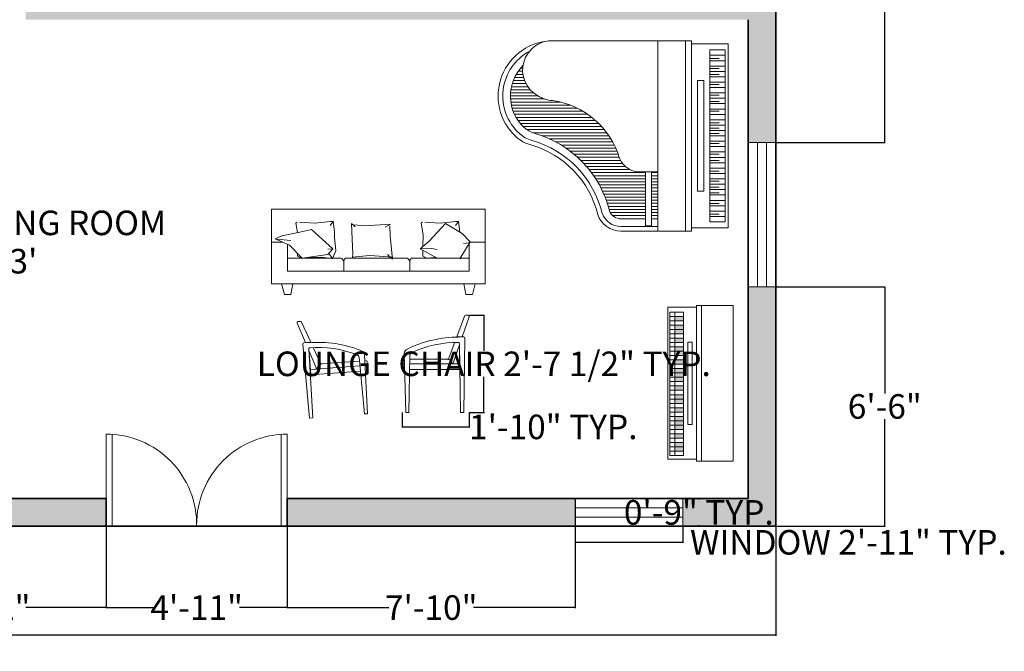
# Model space of a CAD drawing. Units: inches. Extents: x 638 to 1303, y 1 to 699.
# Tile 8 of 21: x 982 to 1303, y 1 to 207. Entities that reach past the tile are written whole.
import ezdxf

# ---------------------------------------------------------------- set-up
doc = ezdxf.new("R2010")
doc.units = ezdxf.units.IN
doc.header["$MEASUREMENT"] = 0
for name, color, linetype, lineweight in [('A-ANNO-DIMS', 2, 'Continuous', 18), ('A-AREA-IDEN', 7, 'Continuous', 18), ('A-DOOR', 4, 'Continuous', 18), ('A-EQPM', 8, 'Continuous', 15), ('A-EQPM-PATT', 8, 'Continuous', 13), ('A-GLAZ', 4, 'Continuous', 18), ('A-WALL', 7, 'Continuous', 35), ('Furniture', 7, 'Continuous', 15)]:
    doc.layers.add(name, color=color, linetype=linetype, lineweight=lineweight)
doc.layers.add('A-WALL-PATT', color=143, linetype='Continuous', lineweight=13, true_color=0x7aafdf)
doc.styles.get("Standard").update_dxf_attribs({"font": 'arial.ttf'})
doc.dimstyles.get("Standard").update_dxf_attribs({"dimtxt": 8, "dimasz": 0.18, "dimexe": 0.18, "dimexo": 0.0625, "dimgap": 0.09, "dimtad": 0, "dimtih": 1, "dimtoh": 1, "dimdec": 4, "dimzin": 0, "dimdsep": 46, "dimlunit": 3, "dimtxsty": 'Standard', "dimcen": 0.09, "dimadec": 0, "dimazin": 0, "dimtfac": 1, "dimtdec": 4, "dimtofl": 0, "dimtmove": 0, "dimatfit": 3, "dimfxl": 1, "dimtolj": 1, "dimtzin": 0, "dimarcsym": 0})

# ---------------------------------------------------------------- blocks, each defined once
blk = doc.blocks.new('WIN-47')
for p, q in [((47, 9), (0, 9)), ((0, 9), (0, 0)), ((47, 0), (47, 9)), ((0, 6), (47, 6)), ((0, 3), (47, 3)), ((0, 0), (47, 0))]:
    blk.add_line(p, q)
blk = doc.blocks.new('WIN-35')
for p, q in [((35, 9), (0, 9)), ((0, 9), (0, 0)), ((35, 0), (35, 9)), ((0, 6), (35, 6)), ((0, 3), (35, 3)), ((0, 0), (35, 0))]:
    blk.add_line(p, q)
blk = doc.blocks.new('CHAIR-LOUNGE')
for p, q in [((20.36, 31.37, -13.5), (17.84, 24.61, -13.5)), ((19.6, 24.61, -13.5), (21.85, 31.1, -13.5)), ((21.48, 31.62, -13.5), (20.73, 31.62, -13.5)), ((17.18, 22.83, -13.5), (15.04, 17.1, -13.5)), ((17.84, 24.61, -13.5), (17.95, 24.61, -13.5)), ((19.01, 24.61, -13.5), (20.08, 24.61, -13.5)), ((20.08, 0, -13.5), (20.47, 24.21, -13.5)), ((16.53, 15.75, -13.5), (18.7, 22, -13.5)), ((19.09, 0, -13.5), (18.7, 22.44, -13.5)), ((18.7, 22.44, -13.5), (18.7, 13.98, -13.5)), ((0, 16.14, -13.5), (0, 16.93, -13.5)), ((1.18, 0, -13.5), (0.7, 19.2, -13.5)), ((2.16, 0, -13.5), (2.56, 18.65, -13.5)), ((2.56, 17.32, -13.5), (15.12, 17.32, -13.5)), ((0.79, 15.75, -13.5), (0, 15.75, -13.5)), ((2.56, 15.75, -13.5), (18.7, 15.75, -13.5)), ((18.7, 13.98, -13.5), (2.56, 13.98, -13.5)), ((18.7, 15.75, -13.5), (16.53, 15.75, -13.5)), ((2.16, 0, -13.5), (1.18, 0, -13.5)), ((20.08, 0, -13.5), (19.09, 0, -13.5))]:
    blk.add_line(p, q)
for centre, radius, start, end in [((20.73, 31.23, -13.5), 0.394, 90, 159.543), ((21.48, 31.23, -13.5), 0.394, 340.9062, 90), ((18.17, -12.57, -13.5), 37.06, 89.5909, 116.1955), ((18.08, -12.05, -13.5), 34.85, 89.1298, 115.4866), ((18.48, -14.75, -13.5), 39.36, 88.7797, 90.7752), ((18.31, 22.44, -13.5), 0.394, 0, 66.9425), ((20.08, 24.21, -13.5), 0.394, 0, 90), ((2.17, 19.17, -13.5), 1.47, 106.2385, 178.6251), ((1.82, 19.5, -13.5), 1.19, 84.4727, 90.6658), ((3.61, 18.49, -13.5), 1.06, 104.0799, 187.3471), ((0.39, 16.93, -13.5), 0.394, 90, 180), ((0.39, 16.14, -13.5), 0.394, 180, 270), ((18.35, -13.63, -13.5), 36.44, 115.6772, 115.6838), ((14.52, 15.54, -13.5), 1.88, 6.4482, 71.4849)]:
    blk.add_arc(centre, radius, start, end)
blk = doc.blocks.new('*D22')
at = {"layer": 'A-ANNO-DIMS', "color": 0, "lineweight": -2, "transparency": 16777216}
for p, q in [((1162.89, 41.76), (1162.89, 36.39)), ((1197.89, 41.76), (1197.89, 36.39)), ((1163.07, 36.57), (1197.71, 36.57)), ((1197.89, 36.57), (1198.07, 36.57))]:
    blk.add_line(p, q, dxfattribs=at)
at = {"layer": 'A-ANNO-DIMS', "color": 0, "transparency": 16777216}
for points in [[(1163.07, 36.6), (1163.07, 36.54), (1162.89, 36.57)], [(1197.71, 36.6), (1197.71, 36.54), (1197.89, 36.57)]]:
    blk.add_solid(points, dxfattribs=at)
at = {"layer": 'Defpoints', "color": 0, "transparency": 16777216}
for p in [(1162.89, 41.82), (1197.89, 41.82), (1197.89, 36.57)]:
    blk.add_point(p, dxfattribs=at)
at = {"layer": 'A-ANNO-DIMS', "color": 0, "transparency": 16777216, "insert": (1251.89, 36.57), "char_height": 8, "attachment_point": 5}
blk.add_mtext('\\A1;WINDOW 2\'-11" TYP.', dxfattribs=at)
blk = doc.blocks.new('*D23')
at = {"layer": 'A-ANNO-DIMS', "color": 0, "lineweight": -2, "transparency": 16777216}
for p, q in [((1197.96, 50.82), (1203.32, 50.82)), ((1203.14, 50.64), (1203.14, 50.49)), ((1197.96, 41.82), (1203.32, 41.82)), ((1203.14, 42), (1203.14, 42.14))]:
    blk.add_line(p, q, dxfattribs=at)
at = {"layer": 'A-ANNO-DIMS', "color": 0, "transparency": 16777216}
for points in [[(1203.11, 50.64), (1203.17, 50.64), (1203.14, 50.82)], [(1203.11, 42), (1203.17, 42), (1203.14, 41.82)]]:
    blk.add_solid(points, dxfattribs=at)
at = {"layer": 'Defpoints', "color": 0, "transparency": 16777216}
for p in [(1197.89, 50.82), (1203.14, 50.82), (1197.89, 41.82)]:
    blk.add_point(p, dxfattribs=at)
at = {"layer": 'A-ANNO-DIMS', "color": 0, "transparency": 16777216, "insert": (1203.14, 46.32), "char_height": 8, "attachment_point": 5}
blk.add_mtext('\\A1;0\'-9" TYP.', dxfattribs=at)
blk = doc.blocks.new('*D36')
at = {"layer": 'A-ANNO-DIMS', "color": 0, "lineweight": -2, "transparency": 16777216}
for p, q in [((1128.41, 110.53), (1133.27, 110.53)), ((1133.09, 110.35), (1133.09, 98.95)), ((1133.09, 79.09), (1133.09, 90.49)), ((1128.41, 78.91), (1133.27, 78.91))]:
    blk.add_line(p, q, dxfattribs=at)
at = {"layer": 'A-ANNO-DIMS', "color": 0, "transparency": 16777216}
for points in [[(1133.06, 110.35), (1133.12, 110.35), (1133.09, 110.53)], [(1133.06, 79.09), (1133.12, 79.09), (1133.09, 78.91)]]:
    blk.add_solid(points, dxfattribs=at)
at = {"layer": 'Defpoints', "color": 0, "transparency": 16777216}
for p in [(1128.35, 110.53), (1133.09, 110.53), (1128.35, 78.91)]:
    blk.add_point(p, dxfattribs=at)
at = {"layer": 'A-ANNO-DIMS', "color": 0, "transparency": 16777216, "insert": (1133.09, 94.72), "char_height": 8, "attachment_point": 5}
blk.add_mtext('\\A1;LOUNGE CHAIR 2\'-7 1/2" TYP.', dxfattribs=at)
blk = doc.blocks.new('*D37')
at = {"layer": 'A-ANNO-DIMS', "color": 0, "lineweight": -2, "transparency": 16777216}
for p, q in [((1106.45, 78.85), (1106.45, 73.99)), ((1128.35, 78.85), (1128.35, 73.99)), ((1106.63, 74.17), (1128.17, 74.17)), ((1128.35, 74.17), (1128.53, 74.17))]:
    blk.add_line(p, q, dxfattribs=at)
at = {"layer": 'A-ANNO-DIMS', "color": 0, "transparency": 16777216}
for points in [[(1106.63, 74.2), (1106.63, 74.14), (1106.45, 74.17)], [(1128.17, 74.2), (1128.17, 74.14), (1128.35, 74.17)]]:
    blk.add_solid(points, dxfattribs=at)
at = {"layer": 'Defpoints', "color": 0, "transparency": 16777216}
for p in [(1106.45, 78.91), (1128.35, 78.91), (1128.35, 74.17)]:
    blk.add_point(p, dxfattribs=at)
at = {"layer": 'A-ANNO-DIMS', "color": 0, "transparency": 16777216, "insert": (1155.73, 74.17), "char_height": 8, "attachment_point": 5}
blk.add_mtext('\\A1;1\'-10" TYP.', dxfattribs=at)
blk = doc.blocks.new('*D44')
at = {"layer": 'A-ANNO-DIMS', "color": 0, "lineweight": -2, "transparency": 16777216}
for p, q in [((917.77, 50.76), (917.77, 15.14)), ((1010.03, 50.76), (1010.03, 15.14)), ((917.95, 15.32), (943.89, 15.32)), ((1009.85, 15.32), (983.91, 15.32))]:
    blk.add_line(p, q, dxfattribs=at)
at = {"layer": 'A-ANNO-DIMS', "color": 0, "transparency": 16777216}
for points in [[(917.95, 15.35), (917.95, 15.29), (917.77, 15.32)], [(1009.85, 15.35), (1009.85, 15.29), (1010.03, 15.32)]]:
    blk.add_solid(points, dxfattribs=at)
at = {"layer": 'Defpoints', "color": 0, "transparency": 16777216}
for p in [(917.77, 50.82), (1010.03, 50.82), (917.77, 15.32)]:
    blk.add_point(p, dxfattribs=at)
at = {"layer": 'A-ANNO-DIMS', "color": 0, "transparency": 16777216, "insert": (963.9, 15.32), "char_height": 8, "attachment_point": 5}
blk.add_mtext('\\A1;7\'-8 1/2"', dxfattribs=at)
blk = doc.blocks.new('*D45')
at = {"layer": 'A-ANNO-DIMS', "color": 0, "lineweight": -2, "transparency": 16777216}
for p, q in [((1010.03, 50.76), (1010.03, 15.14)), ((1069.03, 50.76), (1069.03, 15.14)), ((1010.21, 15.32), (1025.54, 15.32)), ((1068.85, 15.32), (1053.52, 15.32))]:
    blk.add_line(p, q, dxfattribs=at)
at = {"layer": 'A-ANNO-DIMS', "color": 0, "transparency": 16777216}
for points in [[(1010.21, 15.35), (1010.21, 15.29), (1010.03, 15.32)], [(1068.85, 15.35), (1068.85, 15.29), (1069.03, 15.32)]]:
    blk.add_solid(points, dxfattribs=at)
at = {"layer": 'Defpoints', "color": 0, "transparency": 16777216}
for p in [(1010.03, 50.82), (1069.03, 50.82), (1010.03, 15.32)]:
    blk.add_point(p, dxfattribs=at)
at = {"layer": 'A-ANNO-DIMS', "color": 0, "transparency": 16777216, "insert": (1039.53, 15.32), "char_height": 8, "attachment_point": 5}
blk.add_mtext('\\A1;4\'-11"', dxfattribs=at)
blk = doc.blocks.new('*D46')
at = {"layer": 'A-ANNO-DIMS', "color": 0, "lineweight": -2, "transparency": 16777216}
for p, q in [((1069.03, 50.76), (1069.03, 15.14)), ((1162.89, 50.76), (1162.89, 15.14)), ((1069.21, 15.32), (1102.16, 15.32)), ((1162.71, 15.32), (1129.76, 15.32))]:
    blk.add_line(p, q, dxfattribs=at)
at = {"layer": 'A-ANNO-DIMS', "color": 0, "transparency": 16777216}
for points in [[(1069.21, 15.35), (1069.21, 15.29), (1069.03, 15.32)], [(1162.71, 15.35), (1162.71, 15.29), (1162.89, 15.32)]]:
    blk.add_solid(points, dxfattribs=at)
at = {"layer": 'Defpoints', "color": 0, "transparency": 16777216}
for p in [(1069.03, 50.82), (1162.89, 50.82), (1069.03, 15.32)]:
    blk.add_point(p, dxfattribs=at)
at = {"layer": 'A-ANNO-DIMS', "color": 0, "transparency": 16777216, "insert": (1115.96, 15.32), "char_height": 8, "attachment_point": 5}
blk.add_mtext('\\A1;7\'-10"', dxfattribs=at)
blk = doc.blocks.new('*D47')
at = {"layer": 'A-ANNO-DIMS', "color": 0, "lineweight": -2, "transparency": 16777216}
for p, q in [((1228.3, 119.84), (1263.92, 119.84)), ((1263.74, 119.66), (1263.74, 85)), ((1263.74, 42), (1263.74, 76.65)), ((1228.3, 41.82), (1263.92, 41.82))]:
    blk.add_line(p, q, dxfattribs=at)
at = {"layer": 'A-ANNO-DIMS', "color": 0, "transparency": 16777216}
for points in [[(1263.71, 119.66), (1263.77, 119.66), (1263.74, 119.84)], [(1263.71, 42), (1263.77, 42), (1263.74, 41.82)]]:
    blk.add_solid(points, dxfattribs=at)
at = {"layer": 'Defpoints', "color": 0, "transparency": 16777216}
for p in [(1228.24, 119.84), (1263.74, 119.84), (1228.24, 41.82)]:
    blk.add_point(p, dxfattribs=at)
at = {"layer": 'A-ANNO-DIMS', "color": 0, "transparency": 16777216, "insert": (1263.74, 80.83), "char_height": 8, "attachment_point": 5}
blk.add_mtext('\\A1;6\'-6"', dxfattribs=at)
blk = doc.blocks.new('*D48')
at = {"layer": 'A-ANNO-DIMS', "color": 0, "lineweight": -2, "transparency": 16777216}
for p, q in [((1228.3, 262), (1263.92, 262)), ((1263.74, 261.82), (1263.74, 218.52)), ((1263.74, 167.02), (1263.74, 210.31)), ((1228.3, 166.84), (1263.92, 166.84))]:
    blk.add_line(p, q, dxfattribs=at)
at = {"layer": 'A-ANNO-DIMS', "color": 0, "transparency": 16777216}
for points in [[(1263.71, 261.82), (1263.77, 261.82), (1263.74, 262)], [(1263.71, 167.02), (1263.77, 167.02), (1263.74, 166.84)]]:
    blk.add_solid(points, dxfattribs=at)
at = {"layer": 'Defpoints', "color": 0, "transparency": 16777216}
for p in [(1228.24, 262), (1263.74, 262), (1228.24, 166.84)]:
    blk.add_point(p, dxfattribs=at)
at = {"layer": 'A-ANNO-DIMS', "color": 0, "transparency": 16777216, "insert": (1263.74, 214.42), "char_height": 8, "attachment_point": 5}
blk.add_mtext('\\A1;7\'-11"', dxfattribs=at)
blk = doc.blocks.new('*D72')
at = {"layer": 'A-ANNO-DIMS', "color": 0, "lineweight": -2, "transparency": 16777216}
for p, q in [((697.24, 41.76), (697.24, 6.14)), ((1228.24, 41.76), (1228.24, 6.14)), ((697.42, 6.32), (948.75, 6.32)), ((1228.06, 6.32), (976.73, 6.32))]:
    blk.add_line(p, q, dxfattribs=at)
at = {"layer": 'A-ANNO-DIMS', "color": 0, "transparency": 16777216}
for points in [[(697.42, 6.35), (697.42, 6.29), (697.24, 6.32)], [(1228.06, 6.35), (1228.06, 6.29), (1228.24, 6.32)]]:
    blk.add_solid(points, dxfattribs=at)
at = {"layer": 'Defpoints', "color": 0, "transparency": 16777216}
for p in [(697.24, 41.82), (1228.24, 41.82), (1228.24, 6.32)]:
    blk.add_point(p, dxfattribs=at)
at = {"layer": 'A-ANNO-DIMS', "color": 0, "transparency": 16777216, "insert": (962.74, 6.32), "char_height": 8, "attachment_point": 5}
blk.add_mtext('\\A1;44\'-3"', dxfattribs=at)

msp = doc.modelspace()

# ---------------------------------------------------------------- hatches: boundary and pattern name
at = {"layer": 'A-EQPM-PATT'}
h = msp.add_hatch(dxfattribs=at)
h.set_pattern_fill('ANSI31', color=256, scale=7.99998, angle=-45, style=0)
h.paths.add_polyline_path([(1145.84102, 191.85276), (1145.34085, 191.32389), (1144.86884, 190.76975), (1144.42627, 190.19182), (1144.01435, 189.59167), (1143.63417, 188.97092), (1143.28677, 188.33125), (1142.97309, 187.67439), (1142.69397, 187.00211), (1142.45017, 186.31623), (1142.24235, 185.61861), (1142.07108, 184.91113), (1141.93681, 184.1957), (1141.8399, 183.47426), (1141.78062, 182.74876), (1141.75914, 182.02116), (1141.7755, 181.29342), (1141.82966, 180.56752), (1141.92148, 179.84542), (1142.05071, 179.12906), (1142.217, 178.42039), (1142.4199, 177.72132), (1142.65886, 177.03375), (1142.93323, 176.35952), (1143.24228, 175.70046), (1143.58516, 175.05836), (1143.96096, 174.43495), (1144.36865, 173.83191), (1144.80713, 173.25088), (1145.27522, 172.69342), (1145.77165, 172.16105), (1146.29509, 171.6552), (1146.60656, 171.38394), (1146.93161, 171.12912), (1147.26939, 170.89142), (1147.61898, 170.67146), (1147.97946, 170.46984), (1148.34987, 170.2871), (1148.72921, 170.12372), (1149.11648, 169.98013), (1149.51064, 169.85672), (1149.49873, 169.86009), (1151.19358, 169.3362), (1152.85978, 168.72732), (1154.49307, 168.035), (1156.08928, 167.26101), (1157.64434, 166.40733), (1159.15425, 165.47614), (1160.61518, 164.46983), (1162.02337, 163.39097), (1163.37523, 162.2423), (1164.6673, 161.02678), (1165.89629, 159.7475), (1167.05905, 158.40774), (1168.1526, 157.01093), (1169.17416, 155.56062), (1170.12111, 154.06054), (1170.99102, 152.51451), (1171.78169, 150.92649), (1172.49107, 149.30054), (1173.11737, 147.64081), (1173.65898, 145.95154), (1174.11452, 144.23706), (1174.00961, 144.59968), (1174.07994, 144.4099), (1174.16007, 144.22403), (1174.24978, 144.0426), (1174.34883, 143.86609), (1174.45694, 143.69498), (1174.57382, 143.52974), (1174.69916, 143.37082), (1174.83261, 143.21865), (1174.97381, 143.07364), (1175.12238, 142.93619), (1175.27791, 142.80666), (1175.43998, 142.68543), (1175.60815, 142.5728), (1175.78196, 142.46909), (1175.96094, 142.37459), (1176.14461, 142.28954), (1176.33246, 142.21418), (1176.52398, 142.14872), (1176.71865, 142.09333), (1176.91594, 142.04816), (1177.11533, 142.01333), (1177.31625, 141.98895), (1177.51818, 141.97507), (1177.72055, 141.97174), (1177.75898, 141.97192), (1185.75896, 141.97192), (1185.75896, 157.3124), (1184.83225, 157.3124), (1184.47158, 157.27492), (1184.10947, 157.2557), (1183.74686, 157.25479), (1183.38466, 157.27221), (1183.02381, 157.30789), (1182.66522, 157.36175), (1182.3098, 157.43366), (1181.95847, 157.52342), (1181.61213, 157.63082), (1181.27165, 157.75557), (1180.9379, 157.89736), (1180.61175, 158.05583), (1180.29401, 158.23057), (1179.98551, 158.42113), (1179.68702, 158.62703), (1179.39932, 158.84775), (1179.12313, 159.08271), (1178.85916, 159.33133), (1178.60808, 159.59296), (1178.37054, 159.86694), (1178.14714, 160.15256), (1177.93845, 160.44911), (1177.74501, 160.75581), (1177.5673, 161.0719), (1177.40579, 161.39656), (1177.26088, 161.72896), (1177.32575, 161.54611), (1176.90615, 162.87041), (1176.41782, 164.17093), (1175.86213, 165.44413), (1175.24058, 166.68651), (1174.55488, 167.89467), (1173.80691, 169.06529), (1172.99872, 170.19518), (1172.13252, 171.28124), (1171.21068, 172.32049), (1170.23573, 173.31008), (1169.21034, 174.24732), (1168.13732, 175.12961), (1167.01961, 175.95457), (1165.86027, 176.71991), (1164.66247, 177.42354), (1163.4295, 178.06355), (1162.16473, 178.63817), (1160.87163, 179.14582), (1159.55374, 179.58513), (1158.21467, 179.95489), (1156.85809, 180.25407), (1155.48771, 180.48188), (1155.48771, 180.48188), (1154.9771, 180.52604), (1154.46937, 180.59596), (1153.96583, 180.69148), (1153.46776, 180.81235), (1152.97645, 180.95825), (1152.49314, 181.12882), (1152.01908, 181.32361), (1151.55548, 181.54214), (1151.10353, 181.78383), (1150.66438, 182.04807), (1150.66438, 182.04807), (1150.31772, 182.24965), (1149.97982, 182.46558), (1149.65126, 182.69548), (1149.33263, 182.93895), (1149.02448, 183.19556), (1148.72736, 183.46486), (1148.44178, 183.74638), (1148.16825, 184.03962), (1147.90726, 184.34406), (1147.65925, 184.65917), (1147.42466, 184.9844), (1147.20392, 185.31918), (1146.99739, 185.66291), (1146.80546, 186.015), (1146.62844, 186.37482), (1146.46667, 186.74174), (1146.32041, 187.11513), (1146.18993, 187.49431), (1146.07546, 187.87863), (1145.97719, 188.2674), (1145.8953, 188.65996), (1145.82994, 189.0556), (1145.78122, 189.45363), (1145.74922, 189.85336), (1145.734, 190.25408), (1145.73559, 190.65508), (1145.75398, 191.05566), (1145.78914, 191.45512)])
h = msp.add_hatch(dxfattribs=at)
h.set_pattern_fill('ANSI31', color=256, scale=7.99998, angle=-45, style=0)
h.paths.add_polyline_path([(1187.75896, 141.97192), (1189.75896, 141.97192), (1189.75896, 157.3124), (1187.75896, 157.3124)])
h = msp.add_hatch(color=256, dxfattribs=at)
h.paths.add_polyline_path([(1198.1438, 110.18158), (1195.34326, 110.18158), (1195.34326, 108.76426), (1198.1438, 108.76426)])
h.paths.add_polyline_path([(1195.34326, 107.34694), (1195.34326, 105.92962), (1198.1438, 105.92962), (1198.1438, 107.34694)])
h.paths.add_polyline_path([(1198.1438, 105.92962), (1195.34326, 105.92962), (1195.34326, 104.5123), (1198.1438, 104.5123)])
h.paths.add_polyline_path([(1195.34326, 103.09498), (1195.34326, 101.67766), (1198.1438, 101.67766), (1198.1438, 103.09498)])
h.paths.add_polyline_path([(1195.34326, 100.26034), (1195.34326, 98.84302), (1198.1438, 98.84302), (1198.1438, 100.26034)])
h.paths.add_polyline_path([(1198.1438, 98.84302), (1195.34326, 98.84302), (1195.34326, 97.4257), (1198.1438, 97.4257)])
h.paths.add_polyline_path([(1195.34326, 96.00838), (1195.34326, 94.59106), (1198.1438, 94.59106), (1198.1438, 96.00838)])
h.paths.add_polyline_path([(1195.34326, 93.17374), (1195.34326, 91.75642), (1198.1438, 91.75642), (1198.1438, 93.17374)])
h.paths.add_polyline_path([(1198.1438, 91.75642), (1195.34326, 91.75642), (1195.34326, 90.3391), (1198.1438, 90.3391)])
h.paths.add_polyline_path([(1198.1438, 90.3391), (1195.34326, 90.3391), (1195.34326, 88.92178), (1198.1438, 88.92178)])
h.paths.add_polyline_path([(1198.1438, 86.08714), (1198.1438, 87.50446), (1195.34326, 87.50446), (1195.34326, 86.08714)])
h.paths.add_polyline_path([(1195.34326, 84.66982), (1195.34326, 83.2525), (1198.1438, 83.2525), (1198.1438, 84.66982)])
h.paths.add_polyline_path([(1198.1438, 83.2525), (1195.34326, 83.2525), (1195.34326, 81.83518), (1198.1438, 81.83518)])
h.paths.add_polyline_path([(1195.34326, 80.41786), (1195.34326, 79.00054), (1198.1438, 79.00054), (1198.1438, 80.41786)])
h.paths.add_polyline_path([(1195.34326, 77.58322), (1195.34326, 76.1659), (1198.1438, 76.1659), (1198.1438, 77.58322)])
h.paths.add_polyline_path([(1198.1438, 76.1659), (1195.34326, 76.1659), (1195.34326, 74.74858), (1198.1438, 74.74858)])
h.paths.add_polyline_path([(1198.1438, 74.74858), (1195.34326, 74.74858), (1195.34326, 73.33126), (1198.1438, 73.33126)])
h.paths.add_polyline_path([(1195.34326, 71.91394), (1195.34326, 70.49662), (1198.1438, 70.49662), (1198.1438, 71.91394)])
h.paths.add_polyline_path([(1195.34326, 69.0793), (1195.34326, 67.66198), (1198.1438, 67.66198), (1198.1438, 69.0793)])
h.paths.add_polyline_path([(1198.1438, 67.66198), (1195.34326, 67.66198), (1195.34326, 66.24466), (1198.1438, 66.24466)])
at = {"layer": 'A-WALL-PATT'}
h = msp.add_hatch(color=256, dxfattribs=at)
h.dxf.hatch_style = 1
h.paths.add_polyline_path([(973.34524, 629.81895), (793.35541, 629.81895), (793.35541, 620.81895), (850.23798, 620.81895), (922.23798, 620.81895), (922.23798, 524.81895), (908.94335, 524.81895), (908.94335, 520.31895), (926.73798, 520.31895), (926.73798, 544.31895), (979.3571, 544.31895), (979.3571, 548.81895), (926.73798, 548.81895), (926.73798, 620.81895), (973.34524, 620.81895)])
h.paths.add_polyline_path([(758.35541, 629.81895), (697.23798, 629.81895), (697.23798, 586.77451), (706.23798, 586.77451), (706.23798, 620.81895), (758.35541, 620.81895)])
h.paths.add_polyline_path([(1075.85281, 629.81895), (1003.34524, 629.81895), (1003.34524, 620.81895), (1046.73798, 620.81895), (1046.73798, 560.81895), (1046.73798, 548.81895), (1026.3571, 548.81895), (1026.3571, 544.31895), (1046.73798, 544.31895), (1046.73798, 486.87457), (1051.23798, 486.87457), (1051.23798, 556.31895), (1162.89753, 556.31895), (1162.89753, 560.81895), (1051.23798, 560.81895), (1051.23798, 620.81895), (1075.85281, 620.81895)])
h.paths.add_polyline_path([(1228.23798, 629.81895), (1105.85281, 629.81895), (1105.85281, 620.81895), (1219.23798, 620.81895), (1219.23798, 560.81895), (1197.89753, 560.81895), (1197.89753, 556.31895), (1219.23798, 556.31895), (1219.23798, 498.80084), (1228.23798, 498.80084)])
h.paths.add_polyline_path([(1051.23798, 439.87457), (1046.73798, 439.87457), (1046.73798, 407.81895), (1219.23798, 407.81895), (1219.23798, 381.66175), (1228.23798, 381.66175), (1228.23798, 451.80084), (1219.23798, 451.80084), (1219.23798, 412.31895), (1051.23798, 412.31895)])
h.paths.add_polyline_path([(1228.23798, 346.66175), (1219.23798, 346.66175), (1219.23798, 335.81895), (1046.73798, 335.81895), (1046.73798, 273.56895), (1051.23798, 273.56895), (1051.23798, 331.31895), (1219.23798, 331.31895), (1219.23798, 308.99654), (1228.23798, 308.99654)])
h.paths.add_polyline_path([(1228.23798, 261.99654), (1219.23798, 261.99654), (1219.23798, 211.31895), (1051.23798, 211.31895), (1051.23798, 226.56895), (1046.73798, 226.56895), (1046.73798, 211.31895), (983.84714, 211.31895), (983.84714, 206.81895), (1219.23798, 206.81895), (1219.23798, 166.83987), (1228.23798, 166.83987)])
h.paths.add_polyline_path([(1228.23798, 119.83987), (1219.23798, 119.83987), (1219.23798, 50.81895), (1197.89277, 50.81895), (1197.89277, 41.81895), (1228.23798, 41.81895)])
h.paths.add_polyline_path([(1162.89277, 50.81895), (1069.02949, 50.81895), (1069.02949, 41.81895), (1162.89277, 41.81895)])
h.paths.add_polyline_path([(1010.02949, 50.81895), (941.89631, 50.81895), (917.77455, 50.81895), (917.77455, 41.81895), (941.89631, 41.81895), (1010.02949, 41.81895)])
h.paths.add_polyline_path([(882.77455, 50.81895), (854.73798, 50.81895), (854.73798, 145.50379), (850.23798, 145.50379), (850.23798, 50.81895), (793.49755, 50.81895), (793.49755, 41.81895), (882.77455, 41.81895)])
h.paths.add_polyline_path([(746.49755, 50.81895), (706.23798, 50.81895), (706.23798, 96.57416), (697.23798, 96.57416), (697.23798, 41.81895), (746.49755, 41.81895)])
h.paths.add_polyline_path([(706.23798, 206.81895), (714.01165, 206.81895), (714.01165, 211.31895), (706.23798, 211.31895), (706.23798, 251.21966), (697.23798, 251.21966), (697.23798, 143.57416), (706.23798, 143.57416)])
h.paths.add_polyline_path([(923.84714, 211.31895), (854.73798, 211.31895), (854.73798, 397.8313), (850.23798, 397.8313), (850.23798, 388.31895), (747.9539, 388.31895), (747.9539, 383.81895), (850.23798, 383.81895), (850.23798, 311.81895), (706.23798, 311.81895), (706.23798, 342.78787), (697.23798, 342.78787), (697.23798, 281.21966), (706.23798, 281.21966), (706.23798, 307.31895), (850.23798, 307.31895), (850.23798, 211.31895), (749.01165, 211.31895), (749.01165, 206.81895), (850.23798, 206.81895), (850.23798, 192.50379), (854.73798, 192.50379), (854.73798, 206.81895), (923.84714, 206.81895)])
h.paths.add_polyline_path([(706.23798, 434.70471), (697.23798, 434.70471), (697.23798, 372.78787), (706.23798, 372.78787), (706.23798, 383.81895), (712.9539, 383.81895), (712.9539, 388.31895), (706.23798, 388.31895)])
h.paths.add_polyline_path([(706.23798, 520.31895), (850.23798, 520.31895), (850.23798, 444.8313), (854.73798, 444.8313), (854.73798, 520.31895), (861.94335, 520.31895), (861.94335, 524.81895), (706.23798, 524.81895), (706.23798, 551.77451), (697.23798, 551.77451), (697.23798, 481.70471), (706.23798, 481.70471)])

# ---------------------------------------------------------------- linework, layer by layer
at = {"layer": 'A-DOOR'}
for p, q in [((1010.02949, 50.81895), (1010.02949, 71.81895)), ((1012.02949, 41.81895), (1012.02949, 71.75108)), ((1067.02949, 41.81895), (1067.02949, 71.75106)), ((1069.02949, 50.81895), (1069.02949, 71.81895)), ((1010.02949, 41.81895), (1069.02949, 41.81895))]:
    msp.add_line(p, q, dxfattribs=at)
for centre, radius, start, end in [((1010.02949, 42.31478), 29.50417, 359.0370684, 90), ((1069.02949, 42.32311), 29.49583, 90, 180.0161852)]:
    msp.add_arc(centre, radius, start, end, dxfattribs=at)
at = {"layer": 'A-EQPM'}
for p, q in [((1155.75902, 199.97181), (1200.75893, 199.97181)), ((1189.75896, 137.97193), (1189.75896, 199.97181)), ((1198.75894, 137.97193), (1198.75894, 199.97181)), ((1200.75893, 137.97193), (1200.75893, 199.97181)), ((1200.75893, 198.97181), (1212.75891, 198.97181)), ((1212.75891, 198.97181), (1212.75891, 138.97193)), ((1211.75891, 196.97181), (1206.75892, 196.97181)), ((1206.75892, 140.97193), (1206.75892, 196.97181)), ((1211.75891, 196.97181), (1211.75891, 140.97193)), ((1211.75891, 195.22182), (1206.75892, 195.22182)), ((1211.75891, 193.47182), (1206.75892, 193.47182)), ((1211.75891, 191.72182), (1206.75892, 191.72182)), ((1211.75891, 189.97183), (1206.75892, 189.97183)), ((1202.75893, 186.97183), (1202.75893, 150.97191)), ((1204.75893, 186.97183), (1202.75893, 186.97183)), ((1204.75893, 150.97191), (1204.75893, 186.97183)), ((1211.75891, 188.22183), (1206.75892, 188.22183)), ((1211.75891, 186.47184), (1206.75892, 186.47184)), ((1211.75891, 184.72184), (1206.75892, 184.72184)), ((1211.75891, 182.97184), (1206.75892, 182.97184)), ((1211.75891, 181.22185), (1206.75892, 181.22185)), ((1211.75891, 179.47185), (1206.75892, 179.47185)), ((1211.75891, 177.72185), (1206.75892, 177.72185)), ((1211.75891, 175.97186), (1206.75892, 175.97186)), ((1211.75891, 174.22186), (1206.75892, 174.22186)), ((1211.75891, 172.47186), (1206.75892, 172.47186)), ((1211.75891, 170.72187), (1206.75892, 170.72187)), ((1211.75891, 168.97187), (1206.75892, 168.97187)), ((1211.75891, 167.22187), (1206.75892, 167.22187)), ((1211.75891, 165.47188), (1206.75892, 165.47188)), ((1211.75891, 163.72188), (1206.75892, 163.72188)), ((1211.75891, 161.97188), (1206.75892, 161.97188)), ((1189.75896, 157.3124), (1184.83225, 157.3124)), ((1185.75896, 139.68123), (1185.75896, 157.3124)), ((1187.75896, 157.3124), (1187.75896, 139.68123)), ((1211.75891, 160.22189), (1206.75892, 160.22189)), ((1211.75891, 158.47189), (1206.75892, 158.47189)), ((1211.75891, 156.72189), (1206.75892, 156.72189)), ((1211.75891, 154.9719), (1206.75892, 154.9719)), ((1202.75893, 150.97191), (1204.75893, 150.97191)), ((1211.75891, 153.2219), (1206.75892, 153.2219)), ((1211.75891, 151.47191), (1206.75892, 151.47191)), ((1211.75891, 149.72191), (1206.75892, 149.72191)), ((1211.75891, 147.97191), (1206.75892, 147.97191)), ((1211.75891, 146.22192), (1206.75892, 146.22192)), ((1211.75891, 144.47192), (1206.75892, 144.47192)), ((1185.75896, 141.97192), (1177.75898, 141.97192)), ((1189.75896, 141.97192), (1187.75896, 141.97192)), ((1211.75891, 142.72192), (1206.75892, 142.72192)), ((1189.75896, 139.47193), (1177.75898, 139.47193)), ((1200.75893, 137.97193), (1177.75898, 137.97193)), ((1187.75896, 139.68123), (1185.75896, 139.68123)), ((1212.75891, 138.97193), (1200.75893, 138.97193)), ((1211.75891, 140.97193), (1206.75892, 140.97193)), ((1203.98087, 63.03619), (1203.98087, 113.74319)), ((1198.1438, 111.59767), (1193.68668, 111.59767)), ((1198.1438, 110.18158), (1193.68668, 110.18158)), ((1195.34326, 111.59767), (1195.34326, 64.82734)), ((1198.1438, 108.76426), (1193.68668, 108.76426)), ((1198.1438, 107.34694), (1193.68668, 107.34694)), ((1198.1438, 105.92962), (1193.68668, 105.92962)), ((1198.1438, 104.5123), (1193.68668, 104.5123)), ((1198.1438, 103.09498), (1193.68668, 103.09498)), ((1198.1438, 101.67766), (1193.68668, 101.67766)), ((1198.1438, 100.26034), (1193.68668, 100.26034)), ((1198.1438, 98.84302), (1193.68668, 98.84302)), ((1198.1438, 97.4257), (1193.68668, 97.4257)), ((1198.1438, 96.00838), (1193.68668, 96.00838)), ((1198.1438, 94.59106), (1193.68668, 94.59106)), ((1198.1438, 93.17374), (1193.68668, 93.17374)), ((1198.1438, 91.75642), (1193.68668, 91.75642)), ((1198.1438, 90.3391), (1193.68668, 90.3391)), ((1198.1438, 88.92178), (1193.68668, 88.92178)), ((1198.1438, 87.50446), (1193.68668, 87.50446)), ((1198.1438, 86.08714), (1193.68668, 86.08714)), ((1198.1438, 84.66982), (1193.68668, 84.66982)), ((1198.1438, 83.2525), (1193.68668, 83.2525)), ((1198.1438, 81.83518), (1193.68668, 81.83518)), ((1198.1438, 80.41786), (1193.68668, 80.41786)), ((1198.1438, 79.00054), (1193.68668, 79.00054)), ((1198.1438, 77.58322), (1193.68668, 77.58322)), ((1198.1438, 76.1659), (1193.68668, 76.1659)), ((1198.1438, 74.74858), (1193.68668, 74.74858)), ((1198.1438, 73.33126), (1193.68668, 73.33126)), ((1198.1438, 71.91394), (1193.68668, 71.91394)), ((1198.1438, 70.49662), (1193.68668, 70.49662)), ((1198.1438, 69.0793), (1193.68668, 69.0793)), ((1198.1438, 67.66198), (1193.68668, 67.66198)), ((1198.1438, 66.24466), (1193.68668, 66.24466)), ((1198.1438, 64.82734), (1193.68668, 64.82734))]:
    msp.add_line(p, q, dxfattribs=at)
for points in [[(1206.75892, 194.22182), (1209.75892, 194.22182)], [(1206.75892, 190.97183), (1209.75892, 190.97183)], [(1206.75892, 188.97183), (1209.75892, 188.97183)], [(1206.75892, 185.72184), (1209.75892, 185.72184)], [(1206.75892, 182.22184), (1209.75892, 182.22184)], [(1206.75892, 180.22185), (1209.75892, 180.22185)], [(1206.75892, 176.97185), (1209.75892, 176.97185)], [(1206.75892, 173.22186), (1209.75892, 173.22186)], [(1206.75892, 171.47187), (1209.75892, 171.47187)], [(1206.75892, 169.72187), (1209.75892, 169.72187)], [(1206.75892, 166.47188), (1209.75892, 166.47188)], [(1206.75892, 162.97188), (1209.75892, 162.97188)], [(1206.75892, 160.97189), (1209.75892, 160.97189)], [(1206.75892, 157.47189), (1209.75892, 157.47189)], [(1206.75892, 154.2219), (1209.75892, 154.2219)], [(1206.75892, 152.2219), (1209.75892, 152.2219)], [(1206.75892, 150.47191), (1209.75892, 150.47191)], [(1206.75892, 146.97191), (1209.75892, 146.97191)], [(1206.75892, 143.47192), (1209.75892, 143.47192)], [(1202.40607, 63.62674), (1193.05134, 63.62674), (1193.05134, 113.15264), (1202.40607, 113.15264)], [(1193.68668, 111.59767), (1193.68668, 64.82734)], [(1198.1438, 64.82734), (1198.1438, 111.59767)]]:
    msp.add_lwpolyline(points, dxfattribs=at)
for points in [[(1214.32903, 113.74319), (1214.32903, 63.03619), (1202.40607, 63.03619), (1202.40607, 113.74319)], [(1200.96578, 101.8236), (1200.96578, 74.99991), (1199.61395, 74.99991), (1199.61395, 101.8236)]]:
    msp.add_lwpolyline(points, close=True, dxfattribs=at)
for centre, radius, start, end in [((1155.75902, 181.97184), 17.99996, 90, 227.468398), ((1155.2988, 190.4167), 9.56618, 87.2424719, 241.022972), ((1155.75902, 181.97184), 16.49997, 118.4476634, 227.468398), ((1155.75902, 181.97184), 13.99997, 135.107346, 227.468398), ((1156.10492, 190.59288), 10.12982, 237.514781, 266.5068037), ((1151.82187, 154.19372), 26.54253, 16.0815005, 82.0613986), ((1151.70305, 177.55043), 7.99998, 227.468398, 254.094505), ((1151.70305, 177.55043), 11.99998, 227.468398, 254.094505), ((1151.70305, 177.55043), 10.49998, 227.468398, 254.094505), ((1139.98771, 136.08737), 32.58642, 13.4310384, 74.2717971), ((1139.98771, 136.08737), 35.08641, 13.4310384, 74.2717971), ((1139.98771, 136.08737), 31.08642, 13.4310384, 74.2717971), ((1183.91026, 164.42996), 7.17703, 202.10714, 277.380821), ((1177.68325, 145.85317), 3.88161, 198.840232, 270.5504893), ((1177.68325, 145.85317), 7.88161, 198.840232, 270.5504893), ((1177.68325, 145.85317), 6.38161, 198.840232, 270.5504893)]:
    msp.add_arc(centre, radius, start, end, dxfattribs=at)
at = {"layer": 'A-WALL'}
for p, q in [((1228.23798, 629.81895), (1228.23798, 41.81895)), ((1219.23798, 206.81895), (1219.23798, 50.81895)), ((1010.02949, 50.81895), (941.89631, 50.81895)), ((1010.02949, 50.81895), (1010.02949, 41.81895)), ((1219.23798, 50.81895), (1069.02949, 50.81895)), ((1069.02949, 50.81895), (1069.02949, 41.81895)), ((1228.23798, 41.81895), (941.89631, 41.81895))]:
    msp.add_line(p, q, dxfattribs=at)
at = {"layer": 'Furniture'}
for p, q in [((1063.90951, 145.15201), (1133.57362, 145.15201)), ((1063.90951, 145.15201), (1063.90951, 120.76958)), ((1133.57362, 145.15201), (1133.57362, 120.76958)), ((1071.83084, 140.58086), (1072.33431, 140.91617)), ((1072.36331, 137.46526), (1071.83084, 140.58086)), ((1073.05095, 140.86214), (1078.02524, 140.4871)), ((1076.91629, 138.45644), (1073.10092, 137.61977)), ((1083.89564, 132.13492), (1076.91629, 138.45644)), ((1078.02524, 140.4871), (1084.12579, 141.14342)), ((1084.12579, 141.14342), (1082.99953, 139.83079)), ((1083.19134, 141.04289), (1084.03193, 141.04966)), ((1084.03193, 141.04966), (1084.40735, 137.76808)), ((1090.24468, 135.3244), (1089.96449, 140.45605)), ((1089.96449, 140.45605), (1091.17866, 139.33642)), ((1090.71167, 139.98954), (1094.26077, 139.70963)), ((1094.26077, 139.70963), (1102.66654, 140.17614)), ((1102.66654, 140.17614), (1100.98538, 139.24311)), ((1102.47974, 139.70963), (1102.57314, 136.35073)), ((1112.6526, 140.58086), (1113.15607, 140.91617)), ((1113.30958, 136.73672), (1112.6526, 140.58086)), ((1113.87271, 140.86214), (1118.847, 140.4871)), ((1115.33327, 134.72512), (1120.64266, 140.43711)), ((1118.847, 140.4871), (1124.94755, 141.14342)), ((1120.64266, 140.43711), (1126.08818, 137.17312)), ((1124.94755, 141.14342), (1123.82129, 139.83079)), ((1124.0131, 141.04289), (1124.85369, 141.04966)), ((1124.85369, 141.04966), (1125.22911, 137.76808)), ((1067.33132, 136.41124), (1065.09793, 135.48161)), ((1065.09793, 135.48161), (1069.75083, 133.34344)), ((1065.56322, 135.29568), (1070.21612, 134.92383)), ((1073.10092, 137.61977), (1067.33132, 136.41124)), ((1084.40735, 137.76808), (1084.40735, 135.98665)), ((1084.40735, 135.98665), (1084.87663, 131.4862)), ((1090.43148, 130.65927), (1090.24468, 135.3244)), ((1102.57314, 136.35073), (1103.32032, 128.79321)), ((1113.25815, 132.93478), (1113.30958, 136.73672)), ((1126.08818, 137.17312), (1128.6748, 134.45312)), ((1063.90951, 134.35408), (1067.55157, 134.35408)), ((1069.13432, 133.62675), (1069.13432, 124.94942)), ((1069.75083, 133.34344), (1073.93843, 129.16008)), ((1083.5234, 132.13492), (1082.31365, 132.04195)), ((1082.31365, 130.36861), (1083.89564, 132.13492)), ((1112.33823, 132.14112), (1115.33327, 134.72512)), ((1117.9199, 129.14912), (1112.33823, 132.14112)), ((1112.61051, 132.14112), (1116.01396, 132.27712)), ((1113.21572, 129.79853), (1113.24087, 131.65727)), ((1116.01396, 132.27712), (1117.9199, 132.00512)), ((1128.6748, 134.45312), (1125.27135, 128.87712)), ((1128.26638, 134.18112), (1126.49659, 133.90912)), ((1128.34881, 134.35408), (1128.34881, 124.94942)), ((1128.34881, 134.35408), (1133.57362, 134.35408)), ((1069.13432, 129.12927), (1086.57644, 129.12927)), ((1072.39396, 129.79853), (1072.40604, 130.69093)), ((1073.70793, 129.14221), (1072.39396, 129.79853)), ((1076.242, 129.32973), (1073.70793, 129.14221)), ((1073.93843, 129.16008), (1082.31365, 130.36861)), ((1079.99619, 129.42349), (1076.242, 129.32973)), ((1083.75037, 129.04845), (1079.99619, 129.42349)), ((1083.75037, 129.04845), (1082.60785, 130.69709)), ((1084.87663, 131.4862), (1083.75037, 129.04845)), ((1088.06073, 129.12927), (1108.08956, 129.12927)), ((1090.24468, 129.44633), (1095.94193, 130.00615)), ((1090.33808, 129.35303), (1090.43148, 130.65927)), ((1095.94193, 130.00615), (1103.41372, 129.44633)), ((1103.32032, 128.79321), (1101.73256, 130.37936)), ((1109.57385, 129.12927), (1128.34881, 129.12927)), ((1114.52969, 129.14221), (1113.21572, 129.79853)), ((1117.06376, 129.32973), (1114.52969, 129.14221)), ((1117.55985, 129.34212), (1117.06376, 129.32973)), ((1087.43641, 128.18272), (1087.43641, 124.94942)), ((1108.94953, 128.18272), (1108.94953, 124.94942)), ((1069.13432, 124.94942), (1128.34881, 124.94942)), ((1063.90951, 120.76958), (1133.57362, 120.76958)), ((1067.2261, 120.76958), (1068.12591, 117.28637)), ((1070.88085, 120.76958), (1070.206, 117.28637)), ((1126.60228, 120.76958), (1127.27713, 117.28637)), ((1130.25702, 120.76958), (1129.35722, 117.28637)), ((1068.12591, 117.28637), (1070.206, 117.28637)), ((1127.27713, 117.28637), (1129.35722, 117.28637))]:
    msp.add_line(p, q, dxfattribs=at)
for points, knots in [([(1086.57644, 129.12927), (1086.75772, 129.04599), (1087.13198, 128.81967), (1087.33388, 128.41285), (1087.43873, 128.17751)], [15.247039226, 15.247039226, 15.247039226, 15.247039226, 32.166321825, 53.547434874, 53.547434874, 53.547434874, 53.547434874]), ([(1087.43641, 128.16875), (1087.49049, 128.37353), (1087.61443, 128.74984), (1087.91005, 129.01165), (1088.06073, 129.12927)], [5.353257954, 5.353257954, 5.353257954, 5.353257954, 23.098732649, 39.167876379, 39.167876379, 39.167876379, 39.167876379]), ([(1108.08956, 129.12927), (1108.27083, 129.04599), (1108.6451, 128.81967), (1108.847, 128.41285), (1108.95185, 128.17751)], [15.247039226, 15.247039226, 15.247039226, 15.247039226, 32.166321825, 53.547434874, 53.547434874, 53.547434874, 53.547434874]), ([(1108.94953, 128.16875), (1109.00361, 128.37353), (1109.12755, 128.74984), (1109.42317, 129.01165), (1109.57385, 129.12927)], [5.353257954, 5.353257954, 5.353257954, 5.353257954, 23.098732649, 39.167876379, 39.167876379, 39.167876379, 39.167876379])]:
    msp.add_open_spline(points, degree=3, knots=knots, dxfattribs=at)

# ---------------------------------------------------------------- block references
at = {"layer": 'A-GLAZ', "rotation": 270.0000000000011}
msp.add_blockref('WIN-47', (1219.23803, 166.83942), dxfattribs=at)
at = {"layer": 'A-GLAZ'}
msp.add_blockref('WIN-35', (1162.893, 41.819), dxfattribs=at)
at = {"layer": 'Furniture', "extrusion": (0, 0, -1), "zscale": -1, "rotation": 355.7146868009314}
msp.add_blockref('CHAIR-LOUNGE', (-1096.37539, 78.53388), dxfattribs=at)
at = {"layer": 'Furniture'}
msp.add_blockref('CHAIR-LOUNGE', (1106.455, 78.911), dxfattribs=at)

# ---------------------------------------------------------------- texts
at = {"layer": 'A-AREA-IDEN'}
for s, p in [('DRAWING ROOM', (945.90204, 136.63087)), ("30'X13'", (951.07931, 124.1548))]:
    msp.add_text(s, height=8, dxfattribs=at).set_placement(p)

# ---------------------------------------------------------------- dimensions: what is measured, and where the dimension line sits
at = {"layer": 'A-ANNO-DIMS'}
for base, p1, p2, angle, picture, middle in [((1263.73798, 261.99654), (1228.23798, 166.83987), (1228.23798, 261.99654), 90, '*D48', (1263.73798, 214.4182)), ((1263.73798, 119.83987), (1228.23798, 41.81895), (1228.23798, 119.83987), 90, '*D47', (1263.73798, 80.82941)), ((917.77455, 15.31895), (1010.02949, 50.81895), (917.77455, 50.81895), 180, '*D44', (963.90202, 15.31895)), ((1010.02949, 15.31895), (1069.02949, 50.81895), (1010.02949, 50.81895), 180, '*D45', (1039.52949, 15.31895)), ((1069.02949, 15.31895), (1162.89277, 50.81895), (1069.02949, 50.81895), 180, '*D46', (1115.96113, 15.31895))]:
    dim = msp.add_linear_dim(base=base, p1=p1, p2=p2, angle=angle, dimstyle='Standard', override={"dimdec": 1, "dimlfac": 1, "dimrnd": 0, "dimzin": 1, "dimdsep": 46, "dimlunit": 4, "dimfrac": 2}, dxfattribs=at)
    dim.commit()
    dim.dimension.update_dxf_attribs({"geometry": picture, "text_midpoint": middle})
for base, p1, p2, text, picture, middle in [((1133.0894, 110.5337), (1128.34597, 78.91083), (1128.34597, 110.5337), 'LOUNGE CHAIR <> TYP.', '*D36', (1133.0894, 94.72227)), ((1203.14277, 50.81895), (1197.89277, 41.81895), (1197.89277, 50.81895), '<> TYP.', '*D23', (1203.14277, 46.31895))]:
    dim = msp.add_linear_dim(base=base, p1=p1, p2=p2, angle=90, text=text, dimstyle='Standard', override={"dimdec": 1, "dimlfac": 1, "dimrnd": 0, "dimzin": 1, "dimdsep": 46, "dimlunit": 4, "dimfrac": 2}, dxfattribs=at)
    dim.commit()
    dim.dimension.update_dxf_attribs({"geometry": picture, "text_midpoint": middle})
for base, p1, p2, text, picture, middle in [((1128.34597, 74.1674), (1106.45452, 78.91083), (1128.34597, 78.91083), '<> TYP.', '*D37', (1155.7292, 74.1674)), ((1197.89277, 36.56895), (1162.89277, 41.81895), (1197.89277, 41.81895), 'WINDOW <> TYP.', '*D22', (1251.88719, 36.56895))]:
    dim = msp.add_linear_dim(base=base, p1=p1, p2=p2, text=text, dimstyle='Standard', override={"dimdec": 1, "dimlfac": 1, "dimrnd": 0, "dimzin": 1, "dimdsep": 46, "dimlunit": 4, "dimfrac": 2}, dxfattribs=at)
    dim.commit()
    dim.dimension.update_dxf_attribs({"geometry": picture, "text_midpoint": middle})
dim = msp.add_linear_dim(base=(1228.23798, 6.31895), p1=(697.23798, 41.81895), p2=(1228.23798, 41.81895), dimstyle='Standard', override={"dimdec": 1, "dimlfac": 1, "dimrnd": 0, "dimzin": 1, "dimdsep": 46, "dimlunit": 4, "dimfrac": 2}, dxfattribs=at)
dim.commit()
dim.dimension.update_dxf_attribs({"geometry": '*D72', "text_midpoint": (962.73798, 6.31895)})

doc.saveas('drawing.dxf')
